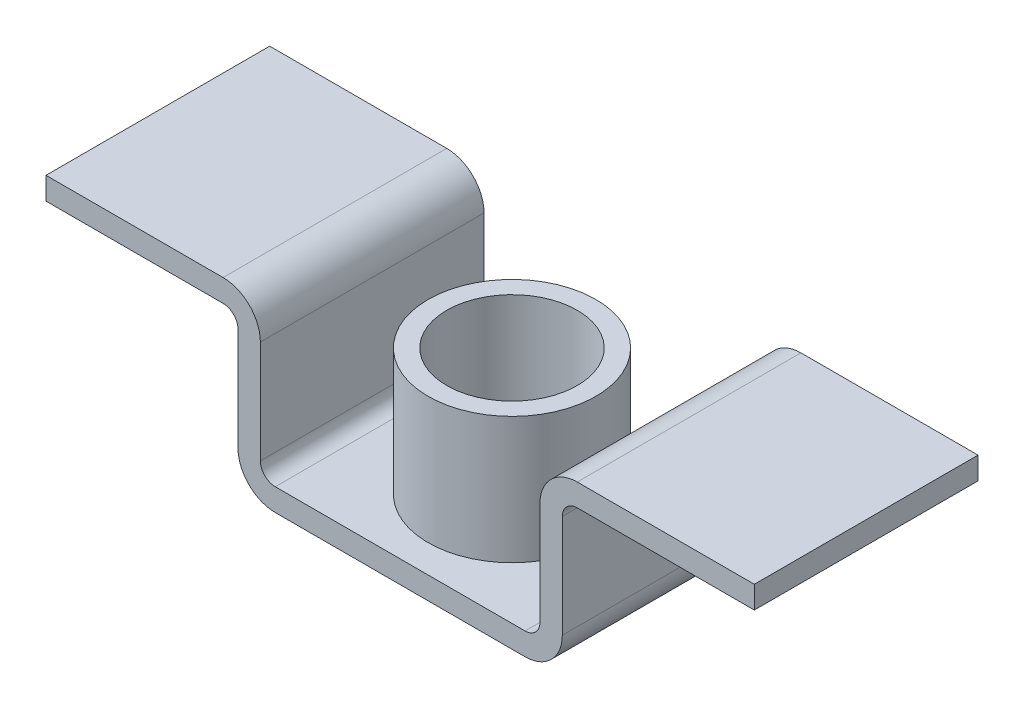
SolidWorks part; units mm, degrees
material "Alloy Steel (SS)"
ref_plane "Front Plane" through (0, 0, 0) normal (0, 0, 1) x (1, 0, 0)
ref_plane "Top Plane" through (0, 0, 0) normal (0, 1, 0) x (1, 0, 0)
ref_plane "Right Plane" through (0, 0, 0) normal (1, 0, 0) x (0, 0, -1)
sketch "Bracket Profile Sketch" plane through (0, 0, 0) normal (0, 0, 1) x (1, 0, 0)
  line L0 (-475, 0) -> (-237.5, 0)
  line L1 (-187.5, -50) -> (-187.5, -188)
  line L2 (-167.5, -208) -> (167.5, -208)
  line L3 (187.5, -188) -> (187.5, -50)
  line L4 (237.5, 0) -> (475, 0)
  line L5 (475, 0) -> (475, -30)
  line L6 (475, -30) -> (237.5, -30)
  line L7 (217.5, -50) -> (217.5, -188)
  line L8 (167.5, -238) -> (-167.5, -238)
  line L9 (-217.5, -188) -> (-217.5, -50)
  line L10 (-237.5, -30) -> (-475, -30)
  line L11 (-475, -30) -> (-475, 0)
  line L12 (0, 0) -> (0, -369.4716) construction
  arc A0 (217.5, -188) -> (167.5, -238) centre (167.5, -188) cw
  arc A1 (187.5, -50) -> (237.5, 0) centre (237.5, -50) cw
  arc A2 (-237.5, 0) -> (-187.5, -50) centre (-237.5, -50) cw
  arc A3 (-167.5, -238) -> (-217.5, -188) centre (-167.5, -188) cw
  arc A4 (237.5, -30) -> (217.5, -50) centre (237.5, -50) ccw
  arc A5 (167.5, -208) -> (187.5, -188) centre (167.5, -188) ccw
  arc A6 (-187.5, -188) -> (-167.5, -208) centre (-167.5, -188) ccw
  arc A7 (-217.5, -50) -> (-237.5, -30) centre (-237.5, -50) ccw
  point P22 (-187.5, 0)
  point P29 (187.5, -208)
  point P32 (-187.5, -208)
  dimension "D7" = 50
  dimension "D8" = 20
  dimension "D1" = 238
  dimension "D2" = 375
  dimension "D3" = 30
  dimension "D4" = 30
  dimension "D5" = 950
  dimension "D6" = 30
extrude "Formed Bracket Body" add sketch "Bracket Profile Sketch" along normal mid plane 300 contours L2 A5 L3 A1 L4 L5 L6 A4 L7 A0 L8 A3 L9 A7 L10 L11 L0 A2 L1 A6
sketch "Boss Tube Sketch" plane through (0, -208, 0) normal (0, 1, 0) x (1, 0, 0)
  circle A0 centre (0, 0) radius 112.5
  circle A1 centre (0, 0) radius 87.5
  dimension "D1" = 225
  dimension "D2" = 175
extrude "Boss Tube Ø225x170" add sketch "Boss Tube Sketch" along normal blind 170
sketch "Base Hole Sketch" plane through (0, -208, 0) normal (0, 1, 0) x (1, 0, 0)
  circle A0 centre (0, 0) radius 37.5
  dimension "D1" = 75
extrude "Base Hole Ø75" cut sketch "Base Hole Sketch" against normal up to next
